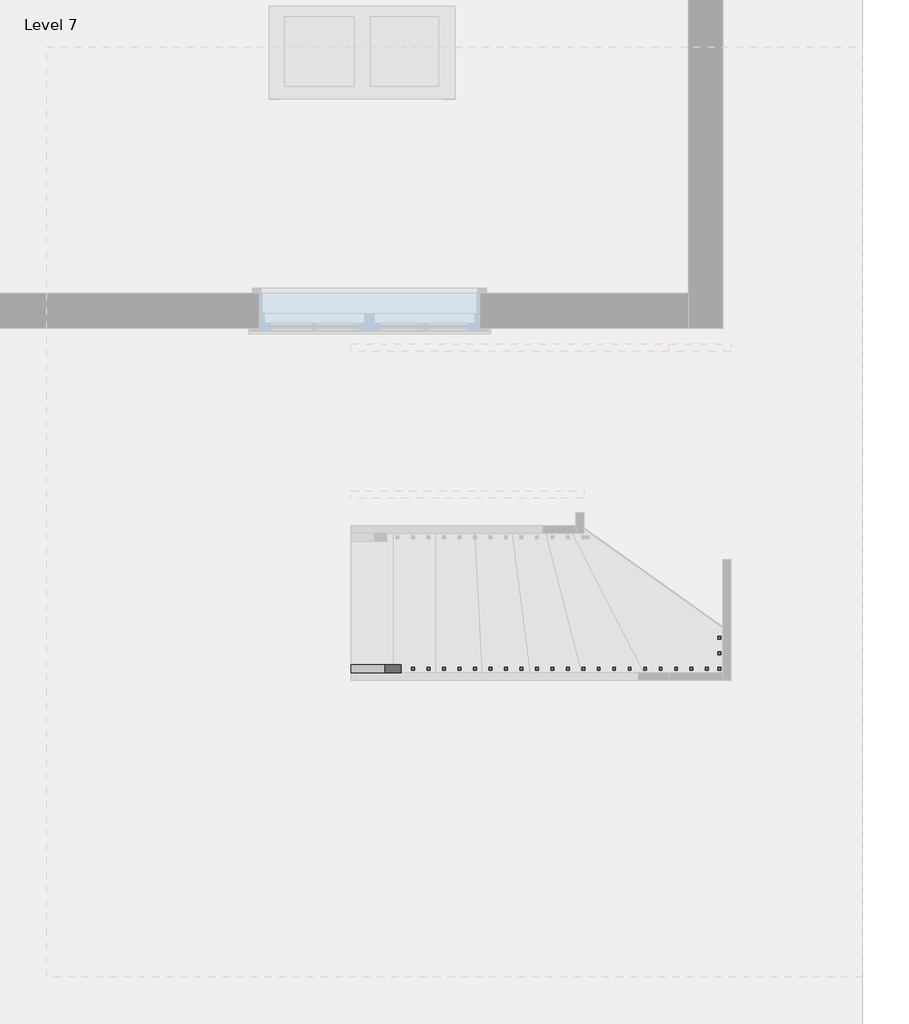
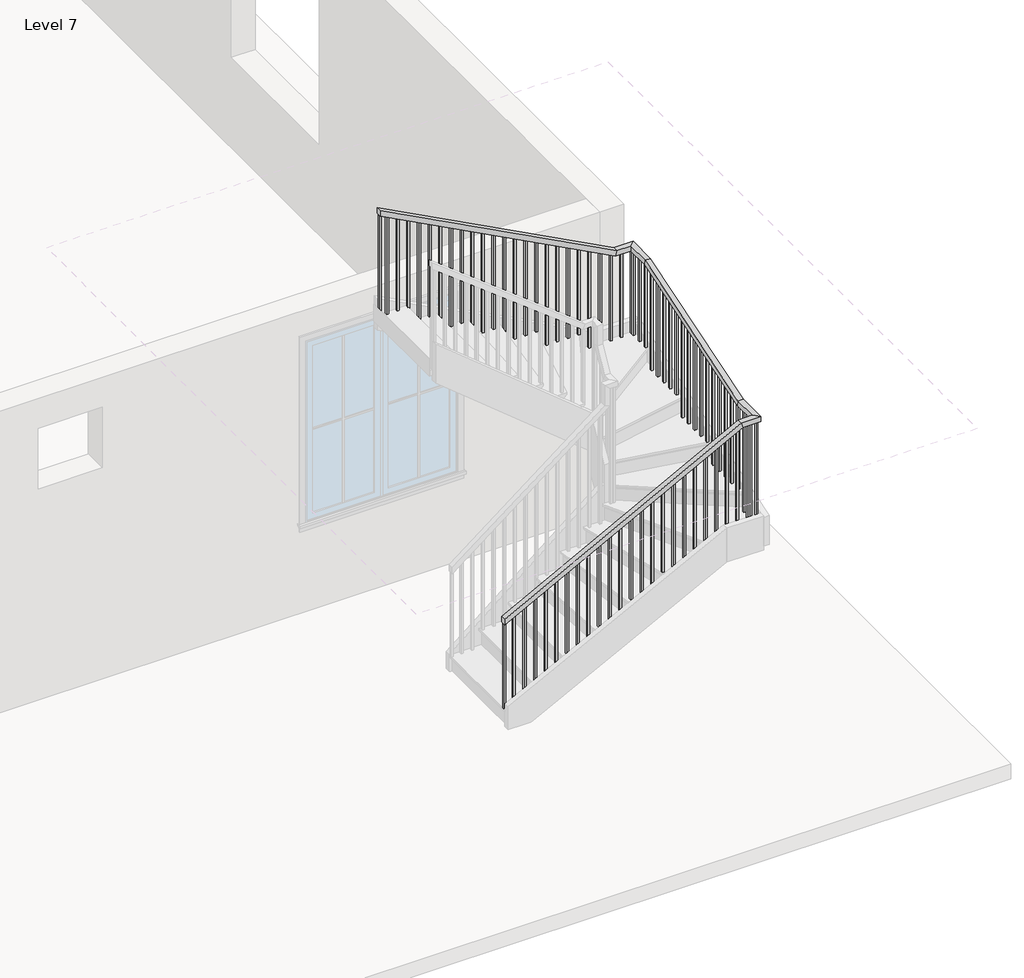
# One storey, part 2 of 3: 1 railing.
"""IFC4 building model written with IfcOpenShell, lengths in millimetres."""

from ifc_helpers import new_model, si_unit, frame, origin, place, context, project, spatial, polyline, outline, extrude, faceted_brep, element, save

model = new_model("IFC4")

# Units and contexts
model_context = context("Model", 3, world=origin())
ifc_project = project(units=[si_unit("LENGTHUNIT", "METRE", prefix="MILLI")], contexts=[model_context])

# Site, building, storey
site = spatial("IfcSite", under=ifc_project)
building = spatial("IfcBuilding", under=site)
storey = spatial("IfcBuildingStorey", under=building, Name="Level 7", Elevation=16002.0)

# Railing
placement = place(None, origin())
element("IfcRailing", 1, ObjectType="Handrail - Rectangular", at=placement, inside=storey, context=model_context, shape_type="SolidModel", body=[
    faceted_brep([(531.7538115, -7514.4090409, 17085.7333333), (531.7538115, -7514.4090409, 17028.2742652), (531.7538115, -7565.2090409, 17028.2742652), (531.7538115, -7565.2090409, 17085.7333333), (2789.4788736, -7514.4090409, 18279.0239201), (2802.0779381, -7514.4090409, 18228.2239201), (2802.0779381, -7565.2090409, 18228.2239201), (2789.4788736, -7565.2090409, 18279.0239201), (2923.0855034, -7269.9465826, 18228.2239201), (2923.0855034, -7277.8971587, 18279.0239201), (2923.0855034, -5744.320923, 18771.1094132), (2923.0855034, -5736.3703469, 18720.3094132), (2973.8855034, -7269.9465826, 18228.2239201), (2973.8855034, -5736.3703469, 18720.3094132), (2973.8855034, -7277.8971587, 18279.0239201), (2973.8855034, -5744.320923, 18771.1094132), (531.7538115, -5507.8090409, 19964.4), (531.7538115, -5457.0090409, 19964.4), (531.7538115, -5457.0090409, 19906.9409318), (531.7538115, -5507.8090409, 19906.9409318), (2776.879809, -5507.8090409, 18720.3094132), (2789.4788736, -5507.8090409, 18771.1094132), (2776.879809, -5457.0090409, 18720.3094132), (2789.4788736, -5457.0090409, 18771.1094132), (2923.0855034, -7514.4090409, 18279.0239201), (2923.0855034, -7514.4090409, 18228.2239201), (2973.8855034, -7565.2090409, 18228.2239201), (2973.8855034, -7565.2090409, 18279.0239201), (2923.0855034, -5507.8090409, 18771.1094132), (2923.0855034, -5507.8090409, 18720.3094132), (2973.8855034, -5457.0090409, 18720.3094132), (2973.8855034, -5457.0090409, 18771.1094132)], [[[0, 1, 2, 3]], [[1, 0, 4, 5]], [[2, 1, 5, 6]], [[3, 2, 6, 7]], [[0, 3, 7, 4]], [[8, 9, 10, 11]], [[12, 8, 11, 13]], [[14, 12, 13, 15]], [[9, 14, 15, 10]], [[16, 17, 18, 19]], [[20, 21, 16, 19]], [[22, 20, 19, 18]], [[23, 22, 18, 17]], [[21, 23, 17, 16]], [[5, 4, 24, 25]], [[6, 5, 25, 26]], [[7, 6, 26, 27]], [[4, 7, 27, 24]], [[25, 24, 9, 8]], [[26, 25, 8, 12]], [[27, 26, 12, 14]], [[24, 27, 14, 9]], [[11, 10, 28, 29]], [[13, 11, 29, 30]], [[15, 13, 30, 31]], [[10, 15, 31, 28]], [[29, 28, 21, 20]], [[30, 29, 20, 22]], [[31, 30, 22, 23]], [[28, 31, 23, 21]]]),
    extrude(outline(polyline([(19859.6597858, 621.2105034), (19869.7284102, 602.1605034), (18880.6666667, 602.1605034), (18880.6666667, 621.2105034), (19859.6597858, 621.2105034)])), frame((0.0, -5491.9340409, 0.0), z_axis=(0.0, 1.0, 0.0), x_axis=(0.0, 0.0, 1.0)), (0.0, 0.0, 1.0), 19.05),
    extrude(outline(polyline([(19805.9604556, 722.8105034), (19816.02908, 703.7605034), (18880.6666667, 703.7605034), (18880.6666667, 722.8105034), (19805.9604556, 722.8105034)])), frame((0.0, -5491.9340409, 0.0), z_axis=(0.0, 1.0, 0.0), x_axis=(0.0, 0.0, 1.0)), (0.0, 0.0, 1.0), 19.05),
    extrude(outline(polyline([(19752.2611254, 824.4105034), (19762.3297498, 805.3605034), (18711.3333333, 805.3605034), (18711.3333333, 824.4105034), (19752.2611254, 824.4105034)])), frame((0.0, -5491.9340409, 0.0), z_axis=(0.0, 1.0, 0.0), x_axis=(0.0, 0.0, 1.0)), (0.0, 0.0, 1.0), 19.05),
    extrude(outline(polyline([(19698.5617952, 926.0105034), (19708.6304196, 906.9605034), (18711.3333333, 906.9605034), (18711.3333333, 926.0105034), (19698.5617952, 926.0105034)])), frame((0.0, -5491.9340409, 0.0), z_axis=(0.0, 1.0, 0.0), x_axis=(0.0, 0.0, 1.0)), (0.0, 0.0, 1.0), 19.05),
    extrude(outline(polyline([(19644.862465, 1027.6105034), (19654.9310894, 1008.5605034), (18711.3333333, 1008.5605034), (18711.3333333, 1027.6105034), (19644.862465, 1027.6105034)])), frame((0.0, -5491.9340409, 0.0), z_axis=(0.0, 1.0, 0.0), x_axis=(0.0, 0.0, 1.0)), (0.0, 0.0, 1.0), 19.05),
    extrude(outline(polyline([(19591.1631348, 1129.2105034), (19601.2317592, 1110.1605034), (18542.0, 1110.1605034), (18542.0, 1129.2105034), (19591.1631348, 1129.2105034)])), frame((0.0, -5491.9340409, 0.0), z_axis=(0.0, 1.0, 0.0), x_axis=(0.0, 0.0, 1.0)), (0.0, 0.0, 1.0), 19.05),
    extrude(outline(polyline([(19537.4638046, 1230.8105034), (19547.532429, 1211.7605034), (18542.0, 1211.7605034), (18542.0, 1230.8105034), (19537.4638046, 1230.8105034)])), frame((0.0, -5491.9340409, 0.0), z_axis=(0.0, 1.0, 0.0), x_axis=(0.0, 0.0, 1.0)), (0.0, 0.0, 1.0), 19.05),
    extrude(outline(polyline([(19483.7644744, 1332.4105034), (19493.8330988, 1313.3605034), (18542.0, 1313.3605034), (18542.0, 1332.4105034), (19483.7644744, 1332.4105034)])), frame((0.0, -5491.9340409, 0.0), z_axis=(0.0, 1.0, 0.0), x_axis=(0.0, 0.0, 1.0)), (0.0, 0.0, 1.0), 19.05),
    extrude(outline(polyline([(19430.0651442, 1434.0105034), (19440.1337686, 1414.9605034), (18372.6666667, 1414.9605034), (18372.6666667, 1434.0105034), (19430.0651442, 1434.0105034)])), frame((0.0, -5491.9340409, 0.0), z_axis=(0.0, 1.0, 0.0), x_axis=(0.0, 0.0, 1.0)), (0.0, 0.0, 1.0), 19.05),
    extrude(outline(polyline([(19376.365814, 1535.6105034), (19386.4344384, 1516.5605034), (18372.6666667, 1516.5605034), (18372.6666667, 1535.6105034), (19376.365814, 1535.6105034)])), frame((0.0, -5491.9340409, 0.0), z_axis=(0.0, 1.0, 0.0), x_axis=(0.0, 0.0, 1.0)), (0.0, 0.0, 1.0), 19.05),
    extrude(outline(polyline([(19322.6664838, 1637.2105034), (19332.7351082, 1618.1605034), (18372.6666667, 1618.1605034), (18372.6666667, 1637.2105034), (19322.6664838, 1637.2105034)])), frame((0.0, -5491.9340409, 0.0), z_axis=(0.0, 1.0, 0.0), x_axis=(0.0, 0.0, 1.0)), (0.0, 0.0, 1.0), 19.05),
    extrude(outline(polyline([(19268.9671536, 1738.8105034), (19279.035778, 1719.7605034), (18203.3333333, 1719.7605034), (18203.3333333, 1738.8105034), (19268.9671536, 1738.8105034)])), frame((0.0, -5491.9340409, 0.0), z_axis=(0.0, 1.0, 0.0), x_axis=(0.0, 0.0, 1.0)), (0.0, 0.0, 1.0), 19.05),
    extrude(outline(polyline([(19215.2678234, 1840.4105034), (19225.3364478, 1821.3605034), (18203.3333333, 1821.3605034), (18203.3333333, 1840.4105034), (19215.2678234, 1840.4105034)])), frame((0.0, -5491.9340409, 0.0), z_axis=(0.0, 1.0, 0.0), x_axis=(0.0, 0.0, 1.0)), (0.0, 0.0, 1.0), 19.05),
    extrude(outline(polyline([(19161.5684932, 1942.0105034), (19171.6371176, 1922.9605034), (18203.3333333, 1922.9605034), (18203.3333333, 1942.0105034), (19161.5684932, 1942.0105034)])), frame((0.0, -5491.9340409, 0.0), z_axis=(0.0, 1.0, 0.0), x_axis=(0.0, 0.0, 1.0)), (0.0, 0.0, 1.0), 19.05),
    extrude(outline(polyline([(19107.869163, 2043.6105034), (19117.9377874, 2024.5605034), (18203.3333333, 2024.5605034), (18203.3333333, 2043.6105034), (19107.869163, 2043.6105034)])), frame((0.0, -5491.9340409, 0.0), z_axis=(0.0, 1.0, 0.0), x_axis=(0.0, 0.0, 1.0)), (0.0, 0.0, 1.0), 19.05),
    extrude(outline(polyline([(19054.1698328, 2145.2105034), (19064.2384572, 2126.1605034), (18034.0, 2126.1605034), (18034.0, 2145.2105034), (19054.1698328, 2145.2105034)])), frame((0.0, -5491.9340409, 0.0), z_axis=(0.0, 1.0, 0.0), x_axis=(0.0, 0.0, 1.0)), (0.0, 0.0, 1.0), 19.05),
    extrude(outline(polyline([(19000.4705026, 2246.8105034), (19010.539127, 2227.7605034), (18034.0, 2227.7605034), (18034.0, 2246.8105034), (19000.4705026, 2246.8105034)])), frame((0.0, -5491.9340409, 0.0), z_axis=(0.0, 1.0, 0.0), x_axis=(0.0, 0.0, 1.0)), (0.0, 0.0, 1.0), 19.05),
    extrude(outline(polyline([(18946.7711724, 2348.4105034), (18956.8397968, 2329.3605034), (18034.0, 2329.3605034), (18034.0, 2348.4105034), (18946.7711724, 2348.4105034)])), frame((0.0, -5491.9340409, 0.0), z_axis=(0.0, 1.0, 0.0), x_axis=(0.0, 0.0, 1.0)), (0.0, 0.0, 1.0), 19.05),
    extrude(outline(polyline([(18893.0718422, 2450.0105034), (18903.1404666, 2430.9605034), (18034.0, 2430.9605034), (18034.0, 2450.0105034), (18893.0718422, 2450.0105034)])), frame((0.0, -5491.9340409, 0.0), z_axis=(0.0, 1.0, 0.0), x_axis=(0.0, 0.0, 1.0)), (0.0, 0.0, 1.0), 19.05),
    extrude(outline(polyline([(18839.372512, 2551.6105034), (18849.4411364, 2532.5605034), (17864.6666667, 2532.5605034), (17864.6666667, 2551.6105034), (18839.372512, 2551.6105034)])), frame((0.0, -5491.9340409, 0.0), z_axis=(0.0, 1.0, 0.0), x_axis=(0.0, 0.0, 1.0)), (0.0, 0.0, 1.0), 19.05),
    extrude(outline(polyline([(18785.6731818, 2653.2105034), (18795.7418062, 2634.1605034), (17864.6666667, 2634.1605034), (17864.6666667, 2653.2105034), (18785.6731818, 2653.2105034)])), frame((0.0, -5491.9340409, 0.0), z_axis=(0.0, 1.0, 0.0), x_axis=(0.0, 0.0, 1.0)), (0.0, 0.0, 1.0), 19.05),
    extrude(outline(polyline([(18731.9738516, 2754.8105034), (18742.042476, 2735.7605034), (17864.6666667, 2735.7605034), (17864.6666667, 2754.8105034), (18731.9738516, 2754.8105034)])), frame((0.0, -5491.9340409, 0.0), z_axis=(0.0, 1.0, 0.0), x_axis=(0.0, 0.0, 1.0)), (0.0, 0.0, 1.0), 19.05),
    extrude(outline(polyline([(2856.4105034, -5472.8840409), (2856.4105034, -5491.9340409), (2837.3605034, -5491.9340409), (2837.3605034, -5472.8840409), (2856.4105034, -5472.8840409)])), frame((0.0, 0.0, 17864.6666667), z_axis=(0.0, 0.0, 1.0), x_axis=(1.0, 0.0, 0.0)), (0.0, 0.0, 1.0), 855.6427466),
    extrude(outline(polyline([(2958.0105034, -5517.3340409), (2938.9605034, -5517.3340409), (2938.9605034, -5498.2840409), (2958.0105034, -5498.2840409), (2958.0105034, -5517.3340409)])), frame((0.0, 0.0, 17864.6666667), z_axis=(0.0, 0.0, 1.0), x_axis=(1.0, 0.0, 0.0)), (0.0, 0.0, 1.0), 855.6427466),
    extrude(outline(polyline([(2958.0105034, -5618.9340409), (2938.9605034, -5618.9340409), (2938.9605034, -5599.8840409), (2958.0105034, -5599.8840409), (2958.0105034, -5618.9340409)])), frame((0.0, 0.0, 17864.6666667), z_axis=(0.0, 0.0, 1.0), x_axis=(1.0, 0.0, 0.0)), (0.0, 0.0, 1.0), 855.6427466),
    extrude(outline(polyline([(2958.0105034, -5720.5340409), (2938.9605034, -5720.5340409), (2938.9605034, -5701.4840409), (2958.0105034, -5701.4840409), (2958.0105034, -5720.5340409)])), frame((0.0, 0.0, 17864.6666667), z_axis=(0.0, 0.0, 1.0), x_axis=(1.0, 0.0, 0.0)), (0.0, 0.0, 1.0), 855.6427466),
    extrude(outline(polyline([(-5822.1340409, 18692.7900316), (-5803.0840409, 18698.9026907), (-5803.0840409, 17695.3333333), (-5822.1340409, 17695.3333333), (-5822.1340409, 18692.7900316)])), frame((2938.9605034, 0.0, 0.0), z_axis=(1.0, 0.0, 0.0), x_axis=(0.0, 1.0, 0.0)), (0.0, 0.0, 1.0), 19.05),
    extrude(outline(polyline([(-5923.7340409, 18660.1891834), (-5904.6840409, 18666.3018425), (-5904.6840409, 17695.3333333), (-5923.7340409, 17695.3333333), (-5923.7340409, 18660.1891834)])), frame((2938.9605034, 0.0, 0.0), z_axis=(1.0, 0.0, 0.0), x_axis=(0.0, 1.0, 0.0)), (0.0, 0.0, 1.0), 19.05),
    extrude(outline(polyline([(-6025.3340409, 18627.5883352), (-6006.2840409, 18633.7009942), (-6006.2840409, 17695.3333333), (-6025.3340409, 17695.3333333), (-6025.3340409, 18627.5883352)])), frame((2938.9605034, 0.0, 0.0), z_axis=(1.0, 0.0, 0.0), x_axis=(0.0, 1.0, 0.0)), (0.0, 0.0, 1.0), 19.05),
    extrude(outline(polyline([(-6126.9340409, 18594.987487), (-6107.8840409, 18601.100146), (-6107.8840409, 17695.3333333), (-6126.9340409, 17695.3333333), (-6126.9340409, 18594.987487)])), frame((2938.9605034, 0.0, 0.0), z_axis=(1.0, 0.0, 0.0), x_axis=(0.0, 1.0, 0.0)), (0.0, 0.0, 1.0), 19.05),
    extrude(outline(polyline([(-6228.5340409, 18562.3866387), (-6209.4840409, 18568.4992978), (-6209.4840409, 17695.3333333), (-6228.5340409, 17695.3333333), (-6228.5340409, 18562.3866387)])), frame((2938.9605034, 0.0, 0.0), z_axis=(1.0, 0.0, 0.0), x_axis=(0.0, 1.0, 0.0)), (0.0, 0.0, 1.0), 19.05),
    extrude(outline(polyline([(-6330.1340409, 18529.7857905), (-6311.0840409, 18535.8984495), (-6311.0840409, 17526.0), (-6330.1340409, 17526.0), (-6330.1340409, 18529.7857905)])), frame((2938.9605034, 0.0, 0.0), z_axis=(1.0, 0.0, 0.0), x_axis=(0.0, 1.0, 0.0)), (0.0, 0.0, 1.0), 19.05),
    extrude(outline(polyline([(-6431.7340409, 18497.1849423), (-6412.6840409, 18503.2976013), (-6412.6840409, 17526.0), (-6431.7340409, 17526.0), (-6431.7340409, 18497.1849423)])), frame((2938.9605034, 0.0, 0.0), z_axis=(1.0, 0.0, 0.0), x_axis=(0.0, 1.0, 0.0)), (0.0, 0.0, 1.0), 19.05),
    extrude(outline(polyline([(-6533.3340409, 18464.584094), (-6514.2840409, 18470.6967531), (-6514.2840409, 17526.0), (-6533.3340409, 17526.0), (-6533.3340409, 18464.584094)])), frame((2938.9605034, 0.0, 0.0), z_axis=(1.0, 0.0, 0.0), x_axis=(0.0, 1.0, 0.0)), (0.0, 0.0, 1.0), 19.05),
    extrude(outline(polyline([(-6634.9340409, 18431.9832458), (-6615.8840409, 18438.0959049), (-6615.8840409, 17526.0), (-6634.9340409, 17526.0), (-6634.9340409, 18431.9832458)])), frame((2938.9605034, 0.0, 0.0), z_axis=(1.0, 0.0, 0.0), x_axis=(0.0, 1.0, 0.0)), (0.0, 0.0, 1.0), 19.05),
    extrude(outline(polyline([(-6736.5340409, 18399.3823976), (-6717.4840409, 18405.4950566), (-6717.4840409, 17526.0), (-6736.5340409, 17526.0), (-6736.5340409, 18399.3823976)])), frame((2938.9605034, 0.0, 0.0), z_axis=(1.0, 0.0, 0.0), x_axis=(0.0, 1.0, 0.0)), (0.0, 0.0, 1.0), 19.05),
    extrude(outline(polyline([(-6838.1340409, 18366.7815494), (-6819.0840409, 18372.8942084), (-6819.0840409, 17356.6666667), (-6838.1340409, 17356.6666667), (-6838.1340409, 18366.7815494)])), frame((2938.9605034, 0.0, 0.0), z_axis=(1.0, 0.0, 0.0), x_axis=(0.0, 1.0, 0.0)), (0.0, 0.0, 1.0), 19.05),
    extrude(outline(polyline([(-6939.7340409, 18334.1807011), (-6920.6840409, 18340.2933602), (-6920.6840409, 17356.6666667), (-6939.7340409, 17356.6666667), (-6939.7340409, 18334.1807011)])), frame((2938.9605034, 0.0, 0.0), z_axis=(1.0, 0.0, 0.0), x_axis=(0.0, 1.0, 0.0)), (0.0, 0.0, 1.0), 19.05),
    extrude(outline(polyline([(-7041.3340409, 18301.5798529), (-7022.2840409, 18307.692512), (-7022.2840409, 17356.6666667), (-7041.3340409, 17356.6666667), (-7041.3340409, 18301.5798529)])), frame((2938.9605034, 0.0, 0.0), z_axis=(1.0, 0.0, 0.0), x_axis=(0.0, 1.0, 0.0)), (0.0, 0.0, 1.0), 19.05),
    extrude(outline(polyline([(-7142.9340409, 18268.9790047), (-7123.8840409, 18275.0916637), (-7123.8840409, 17356.6666667), (-7142.9340409, 17356.6666667), (-7142.9340409, 18268.9790047)])), frame((2938.9605034, 0.0, 0.0), z_axis=(1.0, 0.0, 0.0), x_axis=(0.0, 1.0, 0.0)), (0.0, 0.0, 1.0), 19.05),
    extrude(outline(polyline([(-7244.5340409, 18236.3781565), (-7225.4840409, 18242.4908155), (-7225.4840409, 17356.6666667), (-7244.5340409, 17356.6666667), (-7244.5340409, 18236.3781565)])), frame((2938.9605034, 0.0, 0.0), z_axis=(1.0, 0.0, 0.0), x_axis=(0.0, 1.0, 0.0)), (0.0, 0.0, 1.0), 19.05),
    extrude(outline(polyline([(2958.0105034, -7346.1340409), (2938.9605034, -7346.1340409), (2938.9605034, -7327.0840409), (2958.0105034, -7327.0840409), (2958.0105034, -7346.1340409)])), frame((0.0, 0.0, 17187.3333333), z_axis=(0.0, 0.0, 1.0), x_axis=(1.0, 0.0, 0.0)), (0.0, 0.0, 1.0), 1040.8905868),
    extrude(outline(polyline([(2958.0105034, -7447.7340409), (2938.9605034, -7447.7340409), (2938.9605034, -7428.6840409), (2958.0105034, -7428.6840409), (2958.0105034, -7447.7340409)])), frame((0.0, 0.0, 17187.3333333), z_axis=(0.0, 0.0, 1.0), x_axis=(1.0, 0.0, 0.0)), (0.0, 0.0, 1.0), 1040.8905868),
    extrude(outline(polyline([(2859.0288115, -7549.3340409), (2859.0288115, -7530.2840409), (2878.0788115, -7530.2840409), (2878.0788115, -7549.3340409), (2859.0288115, -7549.3340409)])), frame((0.0, 0.0, 17187.3333333), z_axis=(0.0, 0.0, 1.0), x_axis=(1.0, 0.0, 0.0)), (0.0, 0.0, 1.0), 1040.8905868),
    extrude(outline(polyline([(18214.6938418, 2776.4788115), (18204.6252174, 2757.4288115), (17187.3333333, 2757.4288115), (17187.3333333, 2776.4788115), (18214.6938418, 2776.4788115)])), frame((0.0, -7549.3340409, 0.0), z_axis=(0.0, 1.0, 0.0), x_axis=(0.0, 0.0, 1.0)), (0.0, 0.0, 1.0), 19.05),
    extrude(outline(polyline([(18160.9945116, 2674.8788115), (18150.9258872, 2655.8288115), (17187.3333333, 2655.8288115), (17187.3333333, 2674.8788115), (18160.9945116, 2674.8788115)])), frame((0.0, -7549.3340409, 0.0), z_axis=(0.0, 1.0, 0.0), x_axis=(0.0, 0.0, 1.0)), (0.0, 0.0, 1.0), 19.05),
    extrude(outline(polyline([(18107.2951814, 2573.2788115), (18097.226557, 2554.2288115), (17187.3333333, 2554.2288115), (17187.3333333, 2573.2788115), (18107.2951814, 2573.2788115)])), frame((0.0, -7549.3340409, 0.0), z_axis=(0.0, 1.0, 0.0), x_axis=(0.0, 0.0, 1.0)), (0.0, 0.0, 1.0), 19.05),
    extrude(outline(polyline([(18053.5958512, 2471.6788115), (18043.5272268, 2452.6288115), (17187.3333333, 2452.6288115), (17187.3333333, 2471.6788115), (18053.5958512, 2471.6788115)])), frame((0.0, -7549.3340409, 0.0), z_axis=(0.0, 1.0, 0.0), x_axis=(0.0, 0.0, 1.0)), (0.0, 0.0, 1.0), 19.05),
    extrude(outline(polyline([(17999.896521, 2370.0788115), (17989.8278966, 2351.0288115), (17018.0, 2351.0288115), (17018.0, 2370.0788115), (17999.896521, 2370.0788115)])), frame((0.0, -7549.3340409, 0.0), z_axis=(0.0, 1.0, 0.0), x_axis=(0.0, 0.0, 1.0)), (0.0, 0.0, 1.0), 19.05),
    extrude(outline(polyline([(17946.1971908, 2268.4788115), (17936.1285664, 2249.4288115), (17018.0, 2249.4288115), (17018.0, 2268.4788115), (17946.1971908, 2268.4788115)])), frame((0.0, -7549.3340409, 0.0), z_axis=(0.0, 1.0, 0.0), x_axis=(0.0, 0.0, 1.0)), (0.0, 0.0, 1.0), 19.05),
    extrude(outline(polyline([(17892.4978606, 2166.8788115), (17882.4292362, 2147.8288115), (17018.0, 2147.8288115), (17018.0, 2166.8788115), (17892.4978606, 2166.8788115)])), frame((0.0, -7549.3340409, 0.0), z_axis=(0.0, 1.0, 0.0), x_axis=(0.0, 0.0, 1.0)), (0.0, 0.0, 1.0), 19.05),
    extrude(outline(polyline([(17838.7985304, 2065.2788115), (17828.729906, 2046.2288115), (17018.0, 2046.2288115), (17018.0, 2065.2788115), (17838.7985304, 2065.2788115)])), frame((0.0, -7549.3340409, 0.0), z_axis=(0.0, 1.0, 0.0), x_axis=(0.0, 0.0, 1.0)), (0.0, 0.0, 1.0), 19.05),
    extrude(outline(polyline([(17785.0992002, 1963.6788115), (17775.0305758, 1944.6288115), (16848.6666667, 1944.6288115), (16848.6666667, 1963.6788115), (17785.0992002, 1963.6788115)])), frame((0.0, -7549.3340409, 0.0), z_axis=(0.0, 1.0, 0.0), x_axis=(0.0, 0.0, 1.0)), (0.0, 0.0, 1.0), 19.05),
    extrude(outline(polyline([(17731.39987, 1862.0788115), (17721.3312456, 1843.0288115), (16848.6666667, 1843.0288115), (16848.6666667, 1862.0788115), (17731.39987, 1862.0788115)])), frame((0.0, -7549.3340409, 0.0), z_axis=(0.0, 1.0, 0.0), x_axis=(0.0, 0.0, 1.0)), (0.0, 0.0, 1.0), 19.05),
    extrude(outline(polyline([(17677.7005398, 1760.4788115), (17667.6319154, 1741.4288115), (16848.6666667, 1741.4288115), (16848.6666667, 1760.4788115), (17677.7005398, 1760.4788115)])), frame((0.0, -7549.3340409, 0.0), z_axis=(0.0, 1.0, 0.0), x_axis=(0.0, 0.0, 1.0)), (0.0, 0.0, 1.0), 19.05),
    extrude(outline(polyline([(17624.0012096, 1658.8788115), (17613.9325852, 1639.8288115), (16679.3333333, 1639.8288115), (16679.3333333, 1658.8788115), (17624.0012096, 1658.8788115)])), frame((0.0, -7549.3340409, 0.0), z_axis=(0.0, 1.0, 0.0), x_axis=(0.0, 0.0, 1.0)), (0.0, 0.0, 1.0), 19.05),
    extrude(outline(polyline([(17570.3018794, 1557.2788115), (17560.233255, 1538.2288115), (16679.3333333, 1538.2288115), (16679.3333333, 1557.2788115), (17570.3018794, 1557.2788115)])), frame((0.0, -7549.3340409, 0.0), z_axis=(0.0, 1.0, 0.0), x_axis=(0.0, 0.0, 1.0)), (0.0, 0.0, 1.0), 19.05),
    extrude(outline(polyline([(17516.6025492, 1455.6788115), (17506.5339248, 1436.6288115), (16679.3333333, 1436.6288115), (16679.3333333, 1455.6788115), (17516.6025492, 1455.6788115)])), frame((0.0, -7549.3340409, 0.0), z_axis=(0.0, 1.0, 0.0), x_axis=(0.0, 0.0, 1.0)), (0.0, 0.0, 1.0), 19.05),
    extrude(outline(polyline([(17462.903219, 1354.0788115), (17452.8345946, 1335.0288115), (16510.0, 1335.0288115), (16510.0, 1354.0788115), (17462.903219, 1354.0788115)])), frame((0.0, -7549.3340409, 0.0), z_axis=(0.0, 1.0, 0.0), x_axis=(0.0, 0.0, 1.0)), (0.0, 0.0, 1.0), 19.05),
    extrude(outline(polyline([(17409.2038888, 1252.4788115), (17399.1352644, 1233.4288115), (16510.0, 1233.4288115), (16510.0, 1252.4788115), (17409.2038888, 1252.4788115)])), frame((0.0, -7549.3340409, 0.0), z_axis=(0.0, 1.0, 0.0), x_axis=(0.0, 0.0, 1.0)), (0.0, 0.0, 1.0), 19.05),
    extrude(outline(polyline([(17355.5045586, 1150.8788115), (17345.4359342, 1131.8288115), (16510.0, 1131.8288115), (16510.0, 1150.8788115), (17355.5045586, 1150.8788115)])), frame((0.0, -7549.3340409, 0.0), z_axis=(0.0, 1.0, 0.0), x_axis=(0.0, 0.0, 1.0)), (0.0, 0.0, 1.0), 19.05),
    extrude(outline(polyline([(17301.8052284, 1049.2788115), (17291.736604, 1030.2288115), (16340.6666667, 1030.2288115), (16340.6666667, 1049.2788115), (17301.8052284, 1049.2788115)])), frame((0.0, -7549.3340409, 0.0), z_axis=(0.0, 1.0, 0.0), x_axis=(0.0, 0.0, 1.0)), (0.0, 0.0, 1.0), 19.05),
    extrude(outline(polyline([(17248.1058982, 947.6788115), (17238.0372738, 928.6288115), (16340.6666667, 928.6288115), (16340.6666667, 947.6788115), (17248.1058982, 947.6788115)])), frame((0.0, -7549.3340409, 0.0), z_axis=(0.0, 1.0, 0.0), x_axis=(0.0, 0.0, 1.0)), (0.0, 0.0, 1.0), 19.05),
    extrude(outline(polyline([(17194.406568, 846.0788115), (17184.3379436, 827.0288115), (16340.6666667, 827.0288115), (16340.6666667, 846.0788115), (17194.406568, 846.0788115)])), frame((0.0, -7549.3340409, 0.0), z_axis=(0.0, 1.0, 0.0), x_axis=(0.0, 0.0, 1.0)), (0.0, 0.0, 1.0), 19.05),
    extrude(outline(polyline([(17140.7072378, 744.4788115), (17130.6386134, 725.4288115), (16171.3333333, 725.4288115), (16171.3333333, 744.4788115), (17140.7072378, 744.4788115)])), frame((0.0, -7549.3340409, 0.0), z_axis=(0.0, 1.0, 0.0), x_axis=(0.0, 0.0, 1.0)), (0.0, 0.0, 1.0), 19.05),
    extrude(outline(polyline([(17087.0079076, 642.8788115), (17076.9392831, 623.8288115), (16171.3333333, 623.8288115), (16171.3333333, 642.8788115), (17087.0079076, 642.8788115)])), frame((0.0, -7549.3340409, 0.0), z_axis=(0.0, 1.0, 0.0), x_axis=(0.0, 0.0, 1.0)), (0.0, 0.0, 1.0), 19.05),
    extrude(outline(polyline([(2958.0105034, -5491.9340409), (2938.9605034, -5491.9340409), (2938.9605034, -5472.8840409), (2958.0105034, -5472.8840409), (2958.0105034, -5491.9340409)])), frame((0.0, 0.0, 17864.6666667), z_axis=(0.0, 0.0, 1.0), x_axis=(1.0, 0.0, 0.0)), (0.0, 0.0, 1.0), 855.6427466),
    extrude(outline(polyline([(2938.9605034, -7549.3340409), (2938.9605034, -7530.2840409), (2958.0105034, -7530.2840409), (2958.0105034, -7549.3340409), (2938.9605034, -7549.3340409)])), frame((0.0, 0.0, 17187.3333333), z_axis=(0.0, 0.0, 1.0), x_axis=(1.0, 0.0, 0.0)), (0.0, 0.0, 1.0), 1040.8905868),
    extrude(outline(polyline([(19896.8723074, 550.8038115), (19906.9409318, 531.7538115), (18880.6666667, 531.7538115), (18880.6666667, 550.8038115), (19896.8723074, 550.8038115)])), frame((0.0, -5491.9340409, 0.0), z_axis=(0.0, 1.0, 0.0), x_axis=(0.0, 0.0, 1.0)), (0.0, 0.0, 1.0), 19.05),
    extrude(outline(polyline([(17038.3428896, 550.8038115), (17028.2742652, 531.7538115), (16171.3333333, 531.7538115), (16171.3333333, 550.8038115), (17038.3428896, 550.8038115)])), frame((0.0, -7549.3340409, 0.0), z_axis=(0.0, 1.0, 0.0), x_axis=(0.0, 0.0, 1.0)), (0.0, 0.0, 1.0), 19.05),
])

save(model, "model.ifc")

# Revit data of these elements
# Type "Handrail - Rectangular"
#   Assembly Code = "C2010400"
#   built-in parameter 1008612 = 0.0416667 (stored number, unit not read)
#   built-in parameter 1008611 = 0.0416667 (stored number, unit not read)
#   built-in parameter 1008609 = 0.333333 (stored number, unit not read)
#   built-in parameter 1008604 = 0.166667 (stored number, unit not read)
#   built-in parameter 1008603 = 0.166667 (stored number, unit not read)
#   Railing Height = 3' - 0"
#   built-in parameter 1008630 = 2
#   built-in parameter 1008610 = 2
#   built-in parameter 1008618 = Baluster - Square : 3/4"
# Element 1 (IfcRailing, "Handrail - Rectangular")
#   Phase Created = New Construction
